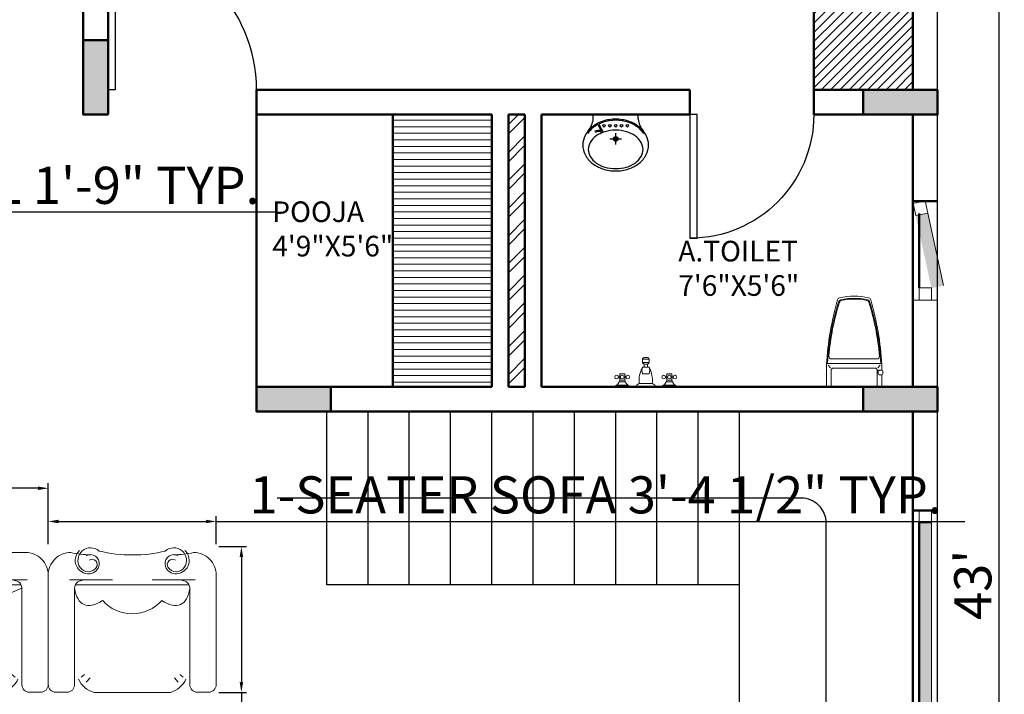
# Model space of a CAD drawing. Units: inches. Extents: x 3064 to 19385, y 846 to 15425.
# Tile 4 of 108: x 3340 to 3579, y 1112 to 1275. Entities that reach past the tile are written whole.
import ezdxf

# ---------------------------------------------------------------- set-up
doc = ezdxf.new("R2010")
doc.units = ezdxf.units.IN
for name, color, linetype, lineweight in [('A-ANNO-DIMS', 2, 'Continuous', 18), ('A-AREA-IDEN', 3, 'Continuous', 18), ('A-COLS', 1, 'Continuous', 35), ('A-DOOR', 3, 'Continuous', 25), ('A-FLOR-FIXT', 9, 'Continuous', 18), ('A-FLOR-STRS', 2, 'Continuous', 25), ('A-FURN', 8, 'Continuous', 18), ('A-FURN-PATT', 252, 'Continuous', 13), ('A-GLAZ', 4, 'Continuous', 18), ('A-WALL', 7, 'Continuous', 50), ('C-PROP', 6, 'Continuous', 25)]:
    doc.layers.add(name, color=color, linetype=linetype, lineweight=lineweight)
doc.layers.add('THIET-BI', color=21, linetype='Continuous')
doc.styles.get("Standard").update_dxf_attribs({"font": 'arial.ttf'})
doc.dimstyles.new('ISO-25', dxfattribs={"dimtxt": 9, "dimasz": 2.5, "dimexe": 1.25, "dimexo": 0.625, "dimtad": 1, "dimdec": 1, "dimlunit": 3, "dimtxsty": 'Standard', "dimcen": 2.5, "dimadec": 0, "dimazin": 0, "dimtfac": 1, "dimtdec": 1, "dimtmove": 0, "dimatfit": 3, "dimfxl": 1, "dimarcsym": 0})

# ---------------------------------------------------------------- blocks, each defined once
blk = doc.blocks.new('*U3')
for p, q in [((0, 0), (0, -6)), ((36, 0), (36, -6))]:
    blk.add_line(p, q)
blk.add_lwpolyline([(0, 0), (0, 36), (1.75, 36), (1.75, 0)], close=True)
blk.add_arc((0, 0), 36, 0, 90)
blk = doc.blocks.new('*U4')
for p, q in [((0, 0), (0, -6)), ((30, 0), (30, -6))]:
    blk.add_line(p, q)
blk.add_lwpolyline([(0, 0), (0, 30), (1.75, 30), (1.75, 0)], close=True)
blk.add_arc((0, 0), 30, 0, 90)
blk = doc.blocks.new('sofa-32')
at = {"color": 0, "linetype": 'ByBlock'}
for p, q in [((-0.026, 0.9238), (-0.1, 0.9238)), ((0.657, 0.9252), (0.1531, 0.9252)), ((1.6158, 0.9252), (2.1197, 0.9252)), ((2.3728, 0.9238), (2.2988, 0.9238)), ((-0.15, 0.15), (-0.15, 0.8738)), ((0.024, 0.2361), (0.024, 0.8738)), ((0.1006, 0.8574), (0.1265, 0.8286)), ((0.7096, 0.8574), (0.6837, 0.8286)), ((0.8227, 0.8633), (0.8259, 0.8195)), ((1.4501, 0.8633), (1.447, 0.8195)), ((1.5632, 0.8574), (1.5891, 0.8286)), ((2.1722, 0.8574), (2.1463, 0.8286)), ((2.2488, 0.2361), (2.2488, 0.8738)), ((2.4228, 0.15), (2.4228, 0.8738)), ((0.05, 0.8375), (0.05, 0.8379)), ((0.0903, 0.8062), (0.0682, 0.8242)), ((0.7199, 0.8062), (0.742, 0.8242)), ((0.7682, 0.3257), (0.7597, 0.8384)), ((0.7601, 0.8375), (0.7601, 0.8379)), ((0.7823, 0.8346), (0.7966, 0.8162)), ((1.4906, 0.8346), (1.4762, 0.8162)), ((1.5046, 0.3257), (1.5131, 0.8384)), ((1.5127, 0.8375), (1.5127, 0.8379)), ((1.5529, 0.8062), (1.5308, 0.8242)), ((2.1825, 0.8062), (2.2046, 0.8242)), ((2.2228, 0.8375), (2.2228, 0.8379)), ((2.2228, 0.8375), (2.2228, 0.8379)), ((0.0289, 0.2145), (2.2439, 0.2145)), ((-0.01, 0.1801), (0.6238, 0.1801)), ((2.2948, 0.1801), (1.661, 0.1801)), ((0, 0), (0.4856, 0)), ((2.2848, 0), (1.7991, 0))]:
    blk.add_line(p, q, dxfattribs=at)
at = {"color": 0, "linetype": 'ByBlock', "extrusion": (0, 0, -1)}
for centre, major_axis, start_param, end_param in [((-0.1, 0.8738), (0.0354, 0.0354), 3.926992, 5.497787), ((-0.026, 0.8738), (-0.0354, 0.0354), 0.785398, 2.356196), ((0.1997, 0.7661), (0.1173, 0.1173), 4.372209, 5.213218), ((0.6105, 0.7661), (0.1173, 0.1173), -0.500829, 0.34018), ((1.6624, 0.7661), (0.1173, 0.1173), 4.372209, 5.213218), ((2.0731, 0.7661), (-0.1173, 0.1173), 1.069968, 1.910976), ((2.2988, 0.8738), (-0.0354, 0.0354), 5.497786, 7.068583), ((2.3728, 0.8738), (0.0354, 0.0354), -0.785398, 0.785398), ((0.8378, 0.8143), (-0.0573, 0.0573), 5.78837, 6.779907), ((1.1202, -2.7856), (2.6094, 2.6094), -0.86827, -0.778364), ((1.1526, -2.7856), (2.6094, 2.6094), -0.792432, -0.702526), ((1.435, 0.8143), (-0.0573, 0.0573), 1.074075, 2.065611), ((0.4599, -0.6685), (0.71, 0.71), 5.048761, 5.844539), ((1.1424, -0.6685), (-0.71, 0.71), 0.438646, 1.125824), ((1.7954, -0.5466), (-0.6249, 0.6249), 0.417642, 1.423136), ((0.074, 0.2361), (0.0354, 0.0354), 2.356194, 3.926992), ((2.1988, 0.2361), (0.0354, 0.0354), 0.785397, 2.356194), ((0, 0.15), (0.1061, 0.1061), 2.356194, 3.926992), ((0.6576, 0.0525), (-0.0624, 0.0624), 4.675944, 7.152385), ((0.6592, 0.0712), (-0.0491, 0.0491), 0.8692, 2.230507), ((1.6256, 0.0712), (-0.0491, 0.0491), 5.623477, 6.984784), ((1.6271, 0.0525), (-0.0624, 0.0624), 0.701599, 3.17804), ((2.2728, 0.15), (0.1061, 0.1061), 0.785398, 2.356194), ((0.6708, 0.0524), (-0.059, 0.059), 3.186406, 6.094039), ((0.6552, 0.0629), (0.0458, 0.0458), 4.523242, 6.472337), ((0.6701, 0.0726), (0.0414, 0.0414), 0.659711, 2.852687), ((0.6801, 0.0798), (-0.0245, 0.0245), 1.759948, 4.523241), ((1.2153, -1.3904), (1.0359, 1.0359), 5.158011, 5.447964), ((1.0694, -1.3904), (1.0359, 1.0359), 5.547613, 5.837566), ((1.6147, 0.0726), (-0.0414, 0.0414), 3.430501, 5.623477), ((1.614, 0.0524), (0.059, 0.059), 0.189149, 3.096782), ((1.6047, 0.0798), (0.0245, 0.0245), 1.759947, 4.52324), ((1.6295, 0.0629), (0.0458, 0.0458), 4.52324, 6.472335), ((0.6324, -0.6613), (-0.479, 0.479), 0.566947, 0.842011), ((1.6523, -0.6613), (0.479, 0.479), 5.441177, 5.716241)]:
    blk.add_ellipse(centre, major_axis=major_axis, ratio=1, start_param=start_param, end_param=end_param, dxfattribs=at)
blk = doc.blocks.new('sofa-34')
at = {"color": 0, "linetype": 'ByBlock'}
for p, q in [((-0.026, 0.9238), (-0.1, 0.9238)), ((0.657, 0.9252), (0.1531, 0.9252)), ((0.8361, 0.9238), (0.9101, 0.9238)), ((-0.15, 0.15), (-0.15, 0.8738)), ((0.024, 0.2361), (0.024, 0.8738)), ((0.1006, 0.8574), (0.1265, 0.8286)), ((0.7096, 0.8574), (0.6837, 0.8286)), ((0.7861, 0.2361), (0.7861, 0.8738)), ((0.9601, 0.15), (0.9601, 0.8738)), ((0.05, 0.8375), (0.05, 0.8379)), ((0.0903, 0.8062), (0.0682, 0.8242)), ((0.7199, 0.8062), (0.742, 0.8242)), ((0.7601, 0.8375), (0.7601, 0.8379)), ((0.7602, 0.8375), (0.7601, 0.8379)), ((0.0289, 0.2145), (0.7812, 0.2145)), ((-0.01, 0.1801), (0.2738, 0.1801)), ((0.8201, 0.1801), (0.5364, 0.1801))]:
    blk.add_line(p, q, dxfattribs=at)
blk.add_arc((0.4051, 0.1479), 0.2579, 40.79835, 139.20165, dxfattribs=at)
at = {"color": 0, "linetype": 'ByBlock', "extrusion": (0, 0, -1)}
for centre, major_axis, ratio, start_param, end_param in [((-0.1, 0.8738), (0.0354, 0.0354), 1, 3.926992, 5.497787), ((-0.026, 0.8738), (-0.0354, 0.0354), 1, 0.785398, 2.356196), ((0.1997, 0.7661), (0.1173, 0.1173), 1, 4.372209, 5.213218), ((0.6105, 0.7661), (0.1173, 0.1173), 1, -0.500829, 0.34018), ((0.5004, -0.5869), (-0.4145, 0.931), 0.264583, -0.381915, 0.387685), ((0.074, 0.2361), (-0.0354, 0.0354), 1, 3.926991, 5.497788), ((0, 0.15), (0.1061, 0.1061), 1, 2.356194, 3.926992), ((0.1167, 0.0525), (-0.0624, 0.0624), 1, 4.675944, 7.152385), ((0.1183, 0.0712), (0.0491, 0.0491), 1, -0.701597, 0.659711), ((0.1299, 0.0524), (-0.059, 0.059), 1, 3.186406, 6.094039), ((0.1144, 0.0629), (-0.0458, 0.0458), 1, 6.094039, 8.043134), ((0.1292, 0.0726), (-0.0414, 0.0414), 1, 2.230507, 4.423483), ((0.1392, 0.0798), (0.0245, 0.0245), 1, 0.189152, 2.952444), ((0.179, -0.6576), (-0.2506, 0.635), 0.885019, 0.124301, 0.339591), ((0.3517, -0.5578), (0.7346, 0.1067), 0.76838, 4.597815, 5.20076)]:
    blk.add_ellipse(centre, major_axis=major_axis, ratio=ratio, start_param=start_param, end_param=end_param, dxfattribs=at)
at = {"color": 0, "linetype": 'ByBlock'}
for centre, major_axis, ratio, start_param, end_param in [((0.8361, 0.8738), (0.0354, 0.0354), 1, 0.785398, 2.356196), ((0.9101, 0.8738), (-0.0354, 0.0354), 1, 3.926992, 5.497787), ((0.3097, -0.5869), (0.4145, 0.931), 0.264583, -0.381915, 0.387685), ((0.7361, 0.2361), (0.0354, 0.0354), 1, 3.926991, 5.497788), ((0.6918, 0.0712), (-0.0491, 0.0491), 1, -0.701597, 0.659711), ((0.6934, 0.0525), (0.0624, 0.0624), 1, 4.675944, 7.152385), ((0.8101, 0.15), (-0.1061, 0.1061), 1, 2.356194, 3.926992), ((0.6809, 0.0726), (0.0414, 0.0414), 1, 2.230507, 4.423483), ((0.6802, 0.0524), (0.059, 0.059), 1, 3.186406, 6.094039), ((0.6709, 0.0798), (-0.0245, 0.0245), 1, 0.189152, 2.952444), ((0.6958, 0.0629), (0.0458, 0.0458), 1, 6.094039, 8.043134), ((0.6312, -0.6576), (0.2506, 0.635), 0.885019, 0.124301, 0.339591)]:
    blk.add_ellipse(centre, major_axis=major_axis, ratio=ratio, start_param=start_param, end_param=end_param, dxfattribs=at)
blk = doc.blocks.new('A$C430D11A0')
at = {"layer": 'THIET-BI'}
for p, q in [((90, 445), (90, 485)), ((475, 485), (90, 485)), ((475, 483), (90, 483)), ((475, 445), (475, 485)), ((129.4, 398.5), (158.2, 344.4)), ((138.3, 403), (176, 332.4)), ((233.4, 275.5), (331.9, 275.5)), ((282.5, 226.2), (282.5, 324.8))]:
    blk.add_line(p, q, dxfattribs=at)
for points in [[(565, 222.5, 0.121635), (544.7, 304.8, 0.10526), (482.3, 379.8, 0.088175), (393.4, 427.4, 0.079002), (282.5, 445, 0.079002), (171.6, 427.4, 0.088175), (82.7, 379.8, 0.10526), (20.3, 304.8, 0.121635), (0, 222.5, 0.121635), (20.3, 140.2, 0.10526), (82.7, 65.2, 0.088175), (171.6, 17.6, 0.079002), (282.5, 0, 0.079002), (393.4, 17.6, 0.088175), (482.3, 65.2, 0.10526), (544.7, 140.2, 0.121635)], [(517.5, 185, 0.134042), (501.2, 244.9, 0.106817), (448.7, 301.7, 0.082468), (375.6, 336.7, 0.070874), (282.5, 350, 0.070874), (189.4, 336.7, 0.082468), (116.3, 301.7, 0.106817), (63.8, 244.9, 0.134042), (47.5, 185, 0.134042), (63.8, 125.1, 0.106817), (116.3, 68.3, 0.082468), (189.4, 33.3, 0.070874), (282.5, 20, 0.070874), (375.6, 33.3, 0.082468), (448.7, 68.3, 0.106817), (501.2, 125.1, 0.134042)]]:
    blk.add_lwpolyline(points, format="xyb", close=True, dxfattribs=at)
for points in [[(522.9, 321.6, 0.07708), (476.1, 372, 0.088175), (390.3, 417.9, 0.079002), (282.5, 435, 0.079002), (174.7, 417.9, 0.035427), (138.3, 403, 0.07708)], [(129.4, 398.5, 0.043566), (88.9, 372, 0.07708), (42.1, 321.6, 0.041486)]]:
    blk.add_lwpolyline(points, format="xyb", dxfattribs=at)
for centre, radius in [((182.5, 388.2), 10.5), ((232.5, 388.2), 10.5), ((282.5, 388.2), 10.5), ((332.5, 388.2), 10.5), ((382.5, 388.2), 10.5), ((282.5, 275.5), 20), ((282.5, 275.5), 15)]:
    blk.add_circle(centre, radius, dxfattribs=at)
for centre, radius, start, end in [((-103.8, 468.9), 195.3, 320.8253, 352.95569), ((668.8, 468.9), 195.3, 187.04431, 219.1747), ((136.4, 285.4), 62.9, 69.64296, 123.47738), ((136.4, 285.4), 52.9, 55.24551, 123.47738)]:
    blk.add_arc(centre, radius, start, end, dxfattribs=at)
blk = doc.blocks.new('WC-P05')
for p, q in [((-202.4, 531.6), (-202.4, 439.1)), ((-192.4, 541.6), (262.6, 541.6)), ((-163.4, 541.6), (-163.4, 400.6)), ((233.6, 541.6), (233.6, 400.6)), ((272.6, 531.6), (272.6, 351.6)), ((-210.4, 430.1), (-210.4, 409.1)), ((-201.4, 439.1), (-180.4, 439.1)), ((-171.4, 430.1), (-171.4, 409.1)), ((-202.4, 400.1), (-202.4, 351.6)), ((-201.4, 400.1), (-180.4, 400.1)), ((-192.4, 341.6), (262.6, 341.6)), ((-166.9, 378.6), (-188.2, 357.3)), ((-143.4, 380.6), (213.6, 380.6)), ((237.1, 378.6), (258.4, 357.3)), ((-159.3, 302.6), (229.5, 302.6))]:
    blk.add_line(p, q)
blk.add_lwpolyline([(-90.9, -221.9, 0.114547), (161, -222, 0.114547)], format="xyb")
for centre, radius, start, end in [((-192.4, 531.6), 10, 90, 180), ((262.6, 531.6), 10, 0, 90), ((-201.4, 430.1), 9, 90, 180), ((-180.4, 430.1), 9, 0, 90), ((-201.4, 409.1), 9, 180, 270), ((2308.9, 492.3), 2515.2, 183.20675, 196.12415), ((-192.4, 351.6), 10, 180, 270), ((1906, 447.2), 2102.6, 182.87428, 197.65536), ((-180.4, 409.1), 9, 270, 0), ((-143.4, 400.6), 20, 180, 270), ((-1835.8, 447.2), 2102.6, 342.34464, 357.12572), ((-2238.7, 492.3), 2515.2, 343.87268, 356.79325), ((213.6, 400.6), 20, 270, 0), ((262.6, 351.6), 10, 270, 0), ((-159.3, 280.1), 22.5, 90, 184.62462), ((1905.9, 447.2), 2094.5, 184.62454, 197.52765), ((-1835.8, 447.2), 2094.6, 342.46396, 355.37538), ((229.5, 280.1), 22.5, 355.37538, 90), ((-85.8, -199.9), 22.5, 196.12415, 256.89941), ((-76.1, -183.7), 22.5, 197.65536, 257.50587), ((-69.9, -176.8), 22.5, 197.52765, 258.10049), ((35.1, 318), 536.4, 257.50587, 282.49413), ((35.7, 324.3), 534.7, 258.10049, 281.73735), ((139.9, -177.1), 22.5, 281.73735, 342.46396), ((146.2, -183.7), 22.5, 282.49413, 342.34464), ((155.9, -200.1), 22.5, 283.03778, 343.87268)]:
    blk.add_arc(centre, radius, start, end)
blk = doc.blocks.new('Faucet - Bathroom front')
for p, q in [((-0.5, 4.25), (0.5, 4.25)), ((0.5, 3.75), (-0.5, 3.75)), ((-0.25, 3), (-0.25, 3.5)), ((0.25, 3.5), (0.25, 3)), ((-4, 1.625), (-4.25, 1.625)), ((-3.25, 1.625), (-3, 1.625)), ((-0.5, 3), (0.5, 3)), ((0.5, 2), (-0.5, 2)), ((3.25, 1.625), (3, 1.625)), ((4, 1.625), (4.25, 1.625)), ((-5, 0), (-2.25, 0)), ((-4.5087, 0.25), (-2.7408, 0.25)), ((-4, 1.375), (-4.25, 1.375)), ((-3.1442, 0.75), (-4.0979, 0.75)), ((-3.25, 1.375), (-3, 1.375)), ((-1.5, 0), (1.5, 0)), ((-1, 0.5), (1, 0.5)), ((2.25, 0), (5, 0)), ((2.7413, 0.25), (4.5092, 0.25)), ((3.25, 1.375), (3, 1.375)), ((4.1058, 0.75), (3.1521, 0.75)), ((4, 1.375), (4.25, 1.375))]:
    blk.add_line(p, q)
for points in [[(-0.5, 3.75), (-0.5, 4.25)], [(-0.25, 4.5), (0.25, 4.5)], [(0.25, 3.5), (-0.25, 3.5)], [(0.5, 4.25), (0.5, 3.75)]]:
    blk.add_lwpolyline(points)
for points in [[(-4, 1), (-4, 2), (-3.25, 2), (-3.25, 1)], [(3.25, 1), (3.25, 2), (4, 2), (4, 1)]]:
    blk.add_lwpolyline(points, close=True)
for centre in [(-4.5, 1.5), (-3.625, 1.5), (-2.75, 1.5), (2.75, 1.5), (3.625, 1.5), (4.5, 1.5)]:
    blk.add_circle(centre, 0.2795)
for centre, radius, start, end in [((-0.2575, 4.2575), 0.2426, 88.22243, 181.7776), ((-0.2575, 3.7425), 0.2426, 178.2224, 271.7776), ((0.2575, 4.2575), 0.2426, 358.2224, 91.77757), ((0.2575, 3.7425), 0.2426, 268.2224, 1.777565), ((3, 1), 4.0311, 150.2551, 187.125), ((0.6413, 2.5), 1.246, 156.3417, 203.6583), ((-3, 1), 4.0311, 352.875, 29.74488), ((-0.6413, 2.5), 1.246, 336.3417, 23.65835), ((-5.375, 1.375), 1.4252, 285.2551, 344.7449), ((-1.875, 1.375), 1.4252, 195.2551, 254.7449), ((-0.7962, -0.2038), 0.7327, 106.1502, 163.8498), ((0.7962, -0.2038), 0.7327, 16.1502, 73.84979), ((1.875, 1.375), 1.4252, 285.2551, 344.7449), ((5.375, 1.375), 1.4252, 195.2551, 254.7449)]:
    blk.add_arc(centre, radius, start, end)
blk = doc.blocks.new('*D42')
at = {"layer": 'A-ANNO-DIMS', "color": 0, "lineweight": -2, "transparency": 16777216}
for p, q in [((3563.47, 1396.34), (3579.02, 1396.34)), ((3577.77, 882.84), (3577.77, 1393.84)), ((3563.47, 880.34), (3579.02, 880.34))]:
    blk.add_line(p, q, dxfattribs=at)
at = {"layer": 'A-ANNO-DIMS', "color": 0, "transparency": 16777216}
for points in [[(3577.35, 1393.84), (3578.19, 1393.84), (3577.77, 1396.34)], [(3577.35, 882.84), (3578.19, 882.84), (3577.77, 880.34)]]:
    blk.add_solid(points, dxfattribs=at)
at = {"layer": 'Defpoints', "color": 0, "transparency": 16777216}
for p in [(3562.85, 1396.34), (3577.77, 1396.34), (3562.85, 880.34)]:
    blk.add_point(p, dxfattribs=at)
at = {"layer": 'A-ANNO-DIMS', "color": 0, "transparency": 16777216, "insert": (3572.55, 1138.34), "char_height": 9, "attachment_point": 5, "rotation": 90}
blk.add_mtext("43'", dxfattribs=at)
blk = doc.blocks.new('WIN-600')
h = blk.add_hatch(color=256)
h.dxf.hatch_style = 1
h.paths.add_polyline_path([(3, 18), (0, 18), (0, 0), (3, 0)])
blk.add_line((3, 18), (3, 0))
blk.add_lwpolyline([(3, 18), (0, 18), (0, 21), (3, 21)], close=True)
blk = doc.blocks.new('WIN-1800-PAIR')
h = blk.add_hatch(color=256)
h.dxf.hatch_style = 1
h.paths.add_polyline_path([(0, 0), (3, 0), (3, 70.5), (0, 70.5)])
h.paths.add_polyline_path([(3, 144), (0, 144), (0, 73.5), (3, 73.5)])
blk.add_line((3, 144), (3, 73.5))
blk.add_lwpolyline([(3, 144), (0, 144), (0, 147), (3, 147)], close=True)
blk = doc.blocks.new('*D409')
at = {"layer": 'A-ANNO-DIMS', "color": 0, "lineweight": -2, "transparency": 16777216}
for p, q in [((3247.88, 1231.24), (3247.88, 1227.47)), ((3268.83, 1231.24), (3268.83, 1227.47)), ((3250.38, 1228.72), (3266.33, 1228.72)), ((3268.83, 1228.72), (3402.5, 1228.72))]:
    blk.add_line(p, q, dxfattribs=at)
at = {"layer": 'A-ANNO-DIMS', "color": 0, "transparency": 16777216}
for points in [[(3250.38, 1229.14), (3250.38, 1228.3), (3247.88, 1228.72)], [(3266.33, 1229.14), (3266.33, 1228.3), (3268.83, 1228.72)]]:
    blk.add_solid(points, dxfattribs=at)
at = {"layer": 'Defpoints', "color": 0, "transparency": 16777216}
for p in [(3247.88, 1231.86), (3268.83, 1231.86), (3268.83, 1228.72)]:
    blk.add_point(p, dxfattribs=at)
at = {"layer": 'A-ANNO-DIMS', "color": 0, "transparency": 16777216, "insert": (3336.92, 1234), "char_height": 9, "attachment_point": 5}
blk.add_mtext('BAR STOOL 1\'-9" TYP.', dxfattribs=at)
blk = doc.blocks.new('*D417')
at = {"layer": 'A-ANNO-DIMS', "color": 0, "lineweight": -2, "transparency": 16777216}
for p, q in [((3253.02, 1148.22), (3253.02, 1162.99)), ((3347.35, 1148.22), (3347.35, 1162.99)), ((3253.02, 1161.74), (3063.75, 1161.74)), ((3344.85, 1161.74), (3255.52, 1161.74))]:
    blk.add_line(p, q, dxfattribs=at)
at = {"layer": 'A-ANNO-DIMS', "color": 0, "transparency": 16777216}
for points in [[(3255.52, 1162.16), (3255.52, 1161.32), (3253.02, 1161.74)], [(3344.85, 1162.16), (3344.85, 1161.32), (3347.35, 1161.74)]]:
    blk.add_solid(points, dxfattribs=at)
at = {"layer": 'Defpoints', "color": 0, "transparency": 16777216}
for p in [(3253.02, 1161.74), (3253.02, 1147.59), (3347.35, 1147.59)]:
    blk.add_point(p, dxfattribs=at)
at = {"layer": 'A-ANNO-DIMS', "color": 0, "transparency": 16777216, "insert": (3157.13, 1167.03), "char_height": 9, "attachment_point": 5}
blk.add_mtext('3-SEATER SOFA 7\'-10 1/2" TYP.', dxfattribs=at)
blk = doc.blocks.new('*D421')
at = {"layer": 'A-ANNO-DIMS', "color": 0, "lineweight": -2, "transparency": 16777216}
for p, q in [((3347.35, 1148.22), (3347.35, 1154.95)), ((3388.05, 1148.22), (3388.05, 1154.95)), ((3349.85, 1153.7), (3385.55, 1153.7)), ((3388.05, 1153.7), (3569.49, 1153.7))]:
    blk.add_line(p, q, dxfattribs=at)
at = {"layer": 'A-ANNO-DIMS', "color": 0, "transparency": 16777216}
for points in [[(3349.85, 1154.11), (3349.85, 1153.28), (3347.35, 1153.7)], [(3385.55, 1154.11), (3385.55, 1153.28), (3388.05, 1153.7)]]:
    blk.add_solid(points, dxfattribs=at)
at = {"layer": 'Defpoints', "color": 0, "transparency": 16777216}
for p in [(3388.05, 1153.7), (3347.35, 1147.59), (3388.05, 1147.59)]:
    blk.add_point(p, dxfattribs=at)
at = {"layer": 'A-ANNO-DIMS', "color": 0, "transparency": 16777216, "insert": (3480.02, 1158.98), "char_height": 9, "attachment_point": 5}
blk.add_mtext('1-SEATER SOFA 3\'-4 1/2" TYP.', dxfattribs=at)
blk = doc.blocks.new('*D422')
at = {"layer": 'A-ANNO-DIMS', "color": 0, "lineweight": -2, "transparency": 16777216}
for p, q in [((3388.68, 1147.59), (3395.41, 1147.59)), ((3394.16, 1145.09), (3394.16, 1114.76)), ((3388.68, 1112.26), (3395.41, 1112.26)), ((3394.16, 1112.26), (3394.16, 1025.53))]:
    blk.add_line(p, q, dxfattribs=at)
at = {"layer": 'A-ANNO-DIMS', "color": 0, "transparency": 16777216}
for points in [[(3393.74, 1145.09), (3394.57, 1145.09), (3394.16, 1147.59)], [(3393.74, 1114.76), (3394.57, 1114.76), (3394.16, 1112.26)]]:
    blk.add_solid(points, dxfattribs=at)
at = {"layer": 'Defpoints', "color": 0, "transparency": 16777216}
for p in [(3388.05, 1147.59), (3388.05, 1112.26), (3394.16, 1112.26)]:
    blk.add_point(p, dxfattribs=at)
at = {"layer": 'A-ANNO-DIMS', "color": 0, "transparency": 16777216, "insert": (3388.88, 1067.64), "char_height": 9, "attachment_point": 5, "rotation": 90}
blk.add_mtext('2\'-11 1/2" TYP.', dxfattribs=at)

msp = doc.modelspace()

# ---------------------------------------------------------------- hatches: boundary and pattern name
at = {"layer": 'A-COLS'}
h = msp.add_hatch(color=256, dxfattribs=at)
h.dxf.hatch_style = 1
h.paths.add_polyline_path([(3355.85, 1252.34), (3361.85, 1252.34), (3361.85, 1270.34), (3355.85, 1270.34)])
h = msp.add_hatch(color=256, dxfattribs=at)
h.dxf.hatch_style = 1
h.paths.add_polyline_path([(3562.85, 1252.34), (3562.85, 1258.34), (3544.85, 1258.34), (3544.85, 1252.34)])
h = msp.add_hatch(color=256, dxfattribs=at)
h.dxf.hatch_style = 1
h.paths.add_polyline_path([(3415.85, 1180.34), (3415.85, 1186.34), (3397.85, 1186.34), (3397.85, 1180.34)])
h = msp.add_hatch(color=256, dxfattribs=at)
h.dxf.hatch_style = 1
h.paths.add_polyline_path([(3562.85, 1180.34), (3562.85, 1186.34), (3544.85, 1186.34), (3544.85, 1180.34)])
at = {"layer": 'A-FURN-PATT'}
h = msp.add_hatch(dxfattribs=at)
h.set_pattern_fill('ANSI31', color=256, scale=0.5)
h.set_pattern_definition([(45, (-2094.8195, 0), (-1.122532, 1.122532), [])])
h.paths.add_polyline_path([(3532.85, 1258.34), (3556.85, 1258.34), (3556.85, 1390.34), (3532.85, 1390.34)])
h = msp.add_hatch(dxfattribs=at)
h.set_pattern_fill('ANSI31', color=256, scale=0.5, angle=135)
h.set_pattern_definition([(180, (-2094.8195, 0), (-1e-16, -1.5875), [])])
h.paths.add_polyline_path([(3430.85, 1186.34), (3454.85, 1186.34), (3454.85, 1252.34), (3430.85, 1252.34)])
h = msp.add_hatch(dxfattribs=at)
h.set_pattern_fill('ANSI32', color=256, scale=0.5)
h.set_pattern_definition([(45, (-2094.8195, 0), (-3.367596, 3.367596), []), (45, (-2092.5745, 0), (-3.367596, 3.367596), [])])
h.paths.add_polyline_path([(3458.85, 1186.34), (3462.85, 1186.34), (3462.85, 1252.34), (3458.85, 1252.34)])

# ---------------------------------------------------------------- linework, layer by layer
at = {"layer": 'A-FLOR-STRS'}
for p, q in [((3414.85, 1138.34), (3414.85, 1180.34)), ((3424.85, 1138.34), (3424.85, 1180.34)), ((3434.85, 1138.34), (3434.85, 1180.34)), ((3444.85, 1138.34), (3444.85, 1180.34)), ((3454.85, 1138.34), (3454.85, 1180.34)), ((3464.85, 1138.34), (3464.85, 1180.34)), ((3474.85, 1138.34), (3474.85, 1180.34)), ((3484.85, 1138.34), (3484.85, 1180.34)), ((3494.85, 1138.34), (3494.85, 1180.34)), ((3504.85, 1138.34), (3504.85, 1180.34)), ((3514.85, 1024.34), (3514.85, 1180.34)), ((3514.85, 1138.34), (3414.85, 1138.34))]:
    msp.add_line(p, q, dxfattribs=at)
msp.add_lwpolyline([(3422.34, 1003.34), (3529.85, 1003.34, 0.414214), (3535.85, 1009.34), (3535.85, 1153.34, 0.414214), (3529.85, 1159.34), (3402.85, 1159.34)], format="xyb", dxfattribs=at)
at = {"layer": 'A-GLAZ'}
msp.add_line((3556.85, 1207.34), (3562.85, 1207.34), dxfattribs=at)
msp.add_lwpolyline([(3561.35, 1207.34), (3558.35, 1207.34), (3558.35, 1210.34), (3561.35, 1210.34)], close=True, dxfattribs=at)
at = {"layer": 'A-WALL'}
for p, q in [((3355.85, 1390.34), (3355.85, 1252.34)), ((3361.85, 1390.34), (3361.85, 1252.34)), ((3532.85, 1252.34), (3532.85, 1390.34)), ((3556.85, 1258.34), (3556.85, 1390.34)), ((3502.85, 1258.34), (3397.85, 1258.34)), ((3397.85, 1258.34), (3397.85, 1180.34)), ((3502.85, 1252.34), (3502.85, 1258.34)), ((3556.85, 1258.34), (3532.85, 1258.34)), ((3361.85, 1252.34), (3355.85, 1252.34)), ((3454.85, 1252.34), (3397.85, 1252.34)), ((3430.85, 1252.34), (3430.85, 1186.34)), ((3454.85, 1252.34), (3454.85, 1186.34)), ((3462.85, 1252.34), (3458.85, 1252.34)), ((3458.85, 1252.34), (3458.85, 1186.34)), ((3462.85, 1186.34), (3462.85, 1252.34)), ((3466.85, 1186.34), (3466.85, 1252.34)), ((3502.85, 1252.34), (3466.85, 1252.34)), ((3556.85, 1252.34), (3532.85, 1252.34)), ((3556.85, 1186.34), (3556.85, 1252.34)), ((3556.85, 1231.34), (3562.85, 1231.34)), ((3558.35, 1228.34), (3558.35, 1210.34)), ((3454.85, 1186.34), (3397.85, 1186.34)), ((3462.85, 1186.34), (3458.85, 1186.34)), ((3556.85, 1186.34), (3466.85, 1186.34)), ((3556.85, 1180.34), (3397.85, 1180.34)), ((3556.85, 982.34), (3556.85, 1180.34)), ((3562.85, 1156.34), (3556.85, 1156.34)), ((3558.35, 1153.34), (3558.35, 1082.84))]:
    msp.add_line(p, q, dxfattribs=at)
for points in [[(3361.85, 1252.34), (3361.85, 1270.34), (3355.85, 1270.34), (3355.85, 1252.34)], [(3562.85, 1258.34), (3544.85, 1258.34), (3544.85, 1252.34), (3562.85, 1252.34)], [(3415.85, 1186.34), (3397.85, 1186.34), (3397.85, 1180.34), (3415.85, 1180.34)], [(3562.85, 1186.34), (3544.85, 1186.34), (3544.85, 1180.34), (3562.85, 1180.34)]]:
    msp.add_lwpolyline(points, close=True, dxfattribs=at)
at = {"layer": 'C-PROP'}
msp.add_line((3562.85, 880.34), (3562.85, 1396.34), dxfattribs=at)

# ---------------------------------------------------------------- block references
at = {"layer": 'A-DOOR'}
msp.add_blockref('*U3', (3361.85, 1258.34), dxfattribs=at)
at = {"layer": 'A-DOOR', "xscale": -1, "rotation": 180}
msp.add_blockref('*U4', (3502.85, 1252.34), dxfattribs=at)
at = {"layer": 'A-FLOR-FIXT'}
for name, p, xscale, yscale, zscale in [('A$C430D11A0', (3476.88, 1238.65), 0.0282220760332506, 0.0282220760332506, 0.0282220760332506), ('Faucet - Bathroom front', (3492.15, 1186.34), 1.573166238287219, 1.573166238287219, 1.573166238287219)]:
    msp.add_blockref(name, p, dxfattribs=dict(at, xscale=xscale, yscale=yscale, zscale=zscale))
at = {"layer": 'A-FLOR-FIXT', "xscale": 0.0282220760332506, "yscale": 0.0282220760332506, "zscale": 0.0282220760332506, "rotation": 180}
msp.add_blockref('WC-P05', (3543.63, 1201.63), dxfattribs=at)
at = {"layer": 'A-FURN', "yscale": 36.66436083614781, "zscale": 36.66436083614781, "rotation": 180}
for name, p, xscale in [('sofa-32', (3341.85, 1146.18), 36.66436083614781), ('sofa-34', (3352.85, 1146.18), -36.66436083614781)]:
    msp.add_blockref(name, p, dxfattribs=dict(at, xscale=xscale))
at = {"layer": 'A-GLAZ', "rotation": 12.21571913413082}
msp.add_blockref('WIN-600', (3561.36, 1210.23), dxfattribs=at)
at = {"layer": 'A-GLAZ'}
msp.add_blockref('WIN-1800-PAIR', (3558.35, 1009.34), dxfattribs=at)

# ---------------------------------------------------------------- texts
at = {"layer": 'A-AREA-IDEN', "char_height": 5, "attachment_point": 1}
for s, insert in [('POOJA\\P4\'9"X5\'6"', (3401.64, 1231.27)), ('A.TOILET\\P7\'6"X5\'6"', (3500.02, 1221.72))]:
    msp.add_mtext_dynamic_manual_height_columns(s, width=67.5924, gutter_width=12.5, heights=[0], dxfattribs=dict(at, insert=insert))

# ---------------------------------------------------------------- dimensions: what is measured, and where the dimension line sits
at = {"layer": 'A-ANNO-DIMS'}
dim = msp.add_linear_dim(base=(3577.77, 1396.34), p1=(3562.85, 880.34), p2=(3562.85, 1396.34), angle=90, dimstyle='ISO-25', override={"dimclrd": 0, "dimclre": 0, "dimclrt": 0}, dxfattribs=at)
dim.commit()
dim.dimension.update_dxf_attribs({"geometry": '*D42', "text_midpoint": (3572.55, 1138.34)})
for base, p1, p2, text, picture, middle in [((3268.8322, 1228.7186), (3247.875, 1231.8622), (3268.8322, 1231.8622), 'BAR STOOL <> TYP.', '*D409', (3336.9156, 1234.0001)), ((3388.05, 1153.7), (3347.35, 1147.59), (3388.05, 1147.59), '1-SEATER SOFA <> TYP.', '*D421', (3480.02, 1158.98))]:
    dim = msp.add_linear_dim(base=base, p1=p1, p2=p2, text=text, dimstyle='ISO-25', override={"dimdec": 1, "dimrnd": 0, "dimzin": 1, "dimlunit": 4, "dimfrac": 2}, dxfattribs=at)
    dim.commit()
    dim.dimension.update_dxf_attribs({"geometry": picture, "text_midpoint": middle})
for base, p1, p2, angle, text, picture, middle in [((3253.02, 1161.74), (3347.35, 1147.59), (3253.02, 1147.59), 180, '3-SEATER SOFA <> TYP.', '*D417', (3157.13, 1167.03)), ((3394.16, 1112.26), (3388.05, 1147.59), (3388.05, 1112.26), 270, '<> TYP.', '*D422', (3388.88, 1067.64))]:
    dim = msp.add_linear_dim(base=base, p1=p1, p2=p2, angle=angle, text=text, dimstyle='ISO-25', override={"dimdec": 1, "dimrnd": 0, "dimzin": 1, "dimlunit": 4, "dimfrac": 2}, dxfattribs=at)
    dim.commit()
    dim.dimension.update_dxf_attribs({"geometry": picture, "text_midpoint": middle})

doc.saveas('drawing.dxf')
